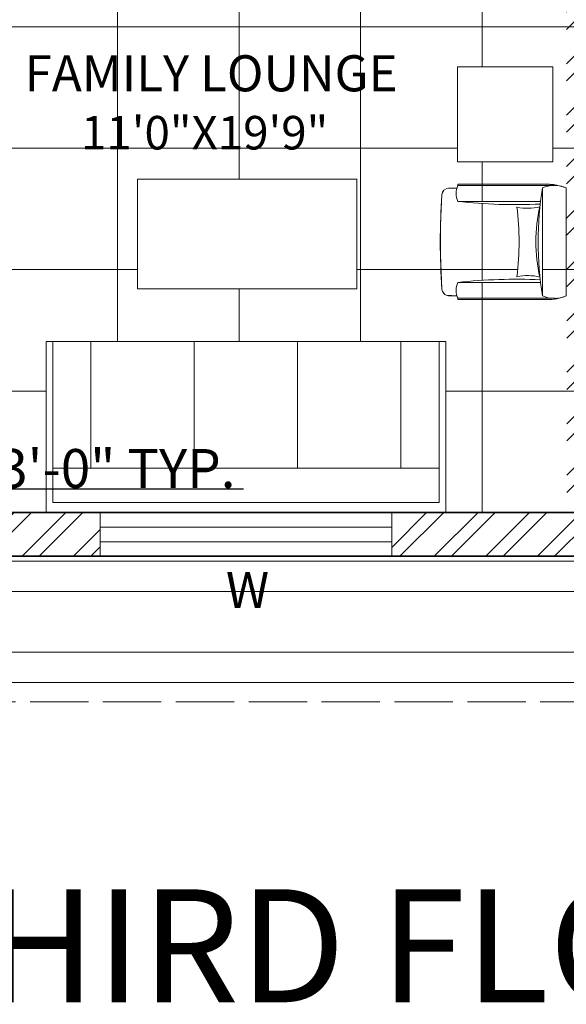
# Model space of a CAD drawing. Units: inches. Extents: x 351 to 1738, y -265 to 286.
# Tile 20 of 38: x 1268 to 1380, y -265 to -63. Entities that reach past the tile are written whole.
import ezdxf

# ---------------------------------------------------------------- set-up
doc = ezdxf.new("R2010")
doc.units = ezdxf.units.IN
doc.header["$MEASUREMENT"] = 0
doc.linetypes.add('ACAD_ISO02W100', pattern=[15, 12, -3])
for name, color, linetype, lineweight in [('A-ANNO-DIMS', 2, 'Continuous', 18), ('A-ANNO-SYMB', 7, 'Continuous', 18), ('A-ANNO-TITL', 7, 'Continuous', 35), ('A-AREA-IDEN', 7, 'Continuous', 18), ('A-FLOR-OVHD', 1, 'ACAD_ISO02W100', 18), ('A-FLOR-PATT', 9, 'Continuous', 9), ('A-FURN', 18, 'Continuous', 13), ('A-GLAZ', 4, 'Continuous', 18), ('A-WALL', 7, 'Continuous', 35), ('A-WALL-PATT', 152, 'Continuous', 13)]:
    doc.layers.add(name, color=color, linetype=linetype, lineweight=lineweight)
doc.styles.add('Annotative', font='arial.ttf')
doc.styles.get("Standard").update_dxf_attribs({"font": 'arial.ttf'})
doc.dimstyles.get("Standard").update_dxf_attribs({"dimtxt": 8, "dimasz": 5, "dimexe": 0.18, "dimexo": 0.0625, "dimgap": 0.09, "dimtad": 1, "dimtoh": 1, "dimzin": 0, "dimdsep": 46, "dimlunit": 4, "dimtxsty": 'Standard', "dimcen": 0, "dimclre": 256, "dimadec": 0, "dimazin": 0, "dimtfac": 1, "dimtofl": 0, "dimtmove": 0, "dimatfit": 3, "dimfxl": 1, "dimtolj": 1, "dimtzin": 0, "dimlwe": -1, "dimarcsym": 0})

# ---------------------------------------------------------------- blocks, each defined once
blk = doc.blocks.new('TABLE-COFFEE-RECT')
blk.add_lwpolyline([(0, 0), (0, 22.55), (45.11, 22.55), (45.11, 0)], close=True)
blk = doc.blocks.new('WIN-60')
for p, q in [((0, 6), (60, 6)), ((0, 3), (60, 3))]:
    blk.add_line(p, q)
blk.add_lwpolyline([(60, 0), (60, 9), (0, 9), (0, 0)], close=True)
blk = doc.blocks.new('*D38')
at = {"layer": 'A-ANNO-DIMS', "color": 0, "lineweight": -2, "transparency": 16777216}
for p, q in [((1215.46, -164.13), (1215.46, -159.13)), ((1215.46, -159.13), (1313.61, -159.13)), ((1215.46, -195.23), (1215.46, -169.13))]:
    blk.add_line(p, q, dxfattribs=at)
at = {"layer": 'A-ANNO-DIMS', "transparency": 16777216}
for p, q in [((1210.11, -164.13), (1215.64, -164.13)), ((1210.11, -200.23), (1215.64, -200.23))]:
    blk.add_line(p, q, dxfattribs=at)
at = {"layer": 'A-ANNO-DIMS', "color": 0, "transparency": 16777216}
for points in [[(1214.63, -169.13), (1216.3, -169.13), (1215.46, -164.13)], [(1214.63, -195.23), (1216.3, -195.23), (1215.46, -200.23)]]:
    blk.add_solid(points, dxfattribs=at)
at = {"layer": 'Defpoints', "color": 0, "transparency": 16777216}
for p in [(1210.05, -164.13), (1215.46, -164.13), (1210.05, -200.23)]:
    blk.add_point(p, dxfattribs=at)
at = {"layer": 'A-ANNO-DIMS', "color": 0, "transparency": 16777216, "insert": (1264.58, -154.96), "char_height": 8, "attachment_point": 5}
blk.add_mtext('\\A1;PLANT B 3\'-0" TYP.', dxfattribs=at)

msp = doc.modelspace()

# ---------------------------------------------------------------- hatches: boundary and pattern name
at = {"layer": 'A-FLOR-PATT', "transparency": 33554559}
h = msp.add_hatch(dxfattribs=at)
h.set_pattern_fill('ANSI37', color=256, scale=200, angle=135)
h.set_pattern_definition([(180, (1112.704, -164.037), (-2e-15, -25), []), (270, (1112.704, -164.037), (25, -5e-15), [])])
h.paths.add_polyline_path([(1380.064, 73.463), (1380.132, 148.463), (1338.064, 148.463), (1290.704, 148.463), (1290.704, 88.463), (1248.704, 88.463), (1248.704, -2.009), (1244.704, -2.009), (1244.704, 142.457), (1160.704, 142.457), (1160.704, 158.963), (1160.704, 170.137), (1160.704, 206.137), (1160.704, 228.963), (1112.704, 228.963), (1112.704, 209.963), (1112.704, 168.963), (1124.704, 168.963), (1124.704, 162.963), (1112.704, 162.963), (1112.704, 64.463), (1112.704, 60.463), (1112.704, 0.463), (1112.704, -48.026), (1146.804, -47.981), (1146.804, -35.691), (1207.804, -35.691), (1207.804, -47.902), (1236.542, -47.864), (1236.544, -50.009), (1248.5, -50.009), (1248.506, -102.915), (1248.512, -150.915), (1248.514, -164.037), (1248.549, -164.037), (1273.017, -164.037), (1273.017, -128.799), (1355.24, -128.799), (1355.24, -164.037), (1384.204, -164.037), (1384.204, -57.037), (1380.064, -57.037), (1380.064, -48.037), (1392.064, -48.037), (1392.064, -53.037), (1406.549, -53.037), (1406.549, -57.037), (1401.204, -57.037), (1401.204, -147.037), (1468.204, -147.037), (1468.204, -138.5), (1472.204, -138.5), (1472.204, -102.5), (1468.204, -102.5), (1468.204, -57.037), (1442.549, -57.037), (1442.549, -53.037), (1463.049, -53.037), (1463.049, -40.747), (1524.049, -40.747), (1524.049, -48.037), (1536.064, -48.037), (1536.064, -53.037), (1557.704, -53.037), (1557.704, 204.963), (1384.204, 204.963), (1384.204, 73.463), (1392.064, 73.463), (1392.064, 64.463), (1384.204, 64.463), (1384.204, -3.5), (1380.204, -3.537), (1380.204, 64.463), (1380.064, 64.463)])
h.paths.add_polyline_path([(1510.714, 86.458, -0.1039845), (1511.661, 85.595, 0.4704384), (1510.158, 87.614, 0.0961001)], flags=16)
h.paths.add_polyline_path([(1510.443, 100.266, 0.009798), (1504.693, 100.48, 0.0287898), (1504.6, 99.767, -0.1653311), (1505.519, 96.135, -0.1436014)], flags=16)
h.paths.add_polyline_path([(1487.201, 85.595, -0.1039845), (1488.148, 86.458, 0.0961001), (1488.704, 87.614, 0.4704384)], flags=0)
h.paths.add_polyline_path([(1495.052, 100.43), (1494.178, 100.43, -0.0264629), (1494.262, 99.774, -0.1442193)], flags=16)
h.paths.add_polyline_path([(1444.485, 86.458, -0.1039845), (1445.433, 85.595, 0.4704384), (1443.93, 87.614, 0.0961001)], flags=16)
h.paths.add_polyline_path([(1420.972, 85.595, -0.1039845), (1421.92, 86.458, 0.0961001), (1422.475, 87.614, 0.4704384)], flags=16)
h.paths.add_polyline_path([(1428.632, 100.335, 0.0010541), (1427.971, 100.309, -0.0215241), (1428.033, 99.774, -0.1143008)], flags=16)
h.paths.add_polyline_path([(1419.906, 143.708, 0.0249793), (1420.222, 157.526), (1421.573, 159.101), (1421.573, 175.369), (1391.393, 175.369), (1391.393, 200.519), (1542.294, 200.519), (1542.294, 175.369), (1512.028, 175.369, 0.0198653), (1511.521, 153.838, 0.0251335), (1512.758, 118.323, 0.0205529), (1512.942, 115.253), (1419.834, 115.253, -0.0004142), (1419.843, 124.798), (1413.059, 124.798), (1413.059, 84.437, -0.0618528), (1415.831, 80.45, -0.0930773), (1420.972, 85.595, -0.2675367), (1422.371, 84.732, 0.0851103), (1424.052, 84.616, -0.8853927), (1424.033, 84.851, -1.1258145), (1424.073, 84.366, -0.0879871), (1422.371, 84.732, -0.2675367), (1422.326, 83.089, -0.3705421), (1420.972, 85.595, 0.0930773), (1415.831, 80.45, -0.0874142), (1417.914, 73.937), (1418.941, 73.937, 0.0272504), (1418.913, 76.906, -0.1157032), (1421.051, 73.937), (1445.354, 73.937, -0.1157032), (1447.492, 76.906, 0.0272504), (1447.464, 73.937), (1448.491, 73.937, -0.0874142), (1450.574, 80.45, 0.0930773), (1445.433, 85.595, -0.3705421), (1444.079, 83.089, -0.2675367), (1444.034, 84.732, -0.0879871), (1442.332, 84.366, -1.1258145), (1442.372, 84.851, -2.0327363), (1442.364, 84.368, 0.0863779), (1444.034, 84.732, -0.2675367), (1445.433, 85.595, -0.0930773), (1450.574, 80.45, -0.2577317), (1466.483, 90.927, -0.4786702), (1468.832, 91.907, -0.4786702), (1471.18, 90.927, -0.26264), (1483.053, 81.78, -0.0718662), (1487.201, 85.595, -0.2675367), (1488.6, 84.732, 0.0851103), (1490.28, 84.616, -0.8853927), (1490.262, 84.851, -1.1258145), (1490.301, 84.366, -0.0879871), (1488.6, 84.732, -0.2675367), (1488.554, 83.089, -0.3705421), (1487.201, 85.595, 0.0718662), (1483.053, 81.78, -0.1320648), (1484.143, 73.937), (1485.169, 73.937, 0.0272504), (1485.142, 76.906, -0.1157032), (1487.28, 73.937), (1511.582, 73.937, -0.1157032), (1513.72, 76.906, 0.0272504), (1513.693, 73.937), (1514.719, 73.937, -0.0874142), (1516.802, 80.45, 0.0930773), (1511.661, 85.595, -0.3705421), (1510.308, 83.089, -0.2675367), (1510.262, 84.732, -0.0879871), (1508.561, 84.366, -1.1258145), (1508.601, 84.851, -2.0327363), (1508.592, 84.368, 0.0863779), (1510.262, 84.732, -0.2675367), (1511.661, 85.595, -0.0930773), (1516.802, 80.45, -0.0618528), (1519.575, 84.437), (1519.575, 73.937), (1413.059, 73.937), (1413.059, 124.798), (1419.843, 124.798, -0.0008205)], flags=16)
h.paths.add_polyline_path([(1220.149, 54.133, -0.1039845), (1220.869, 53.476, 0.4704384), (1219.727, 55.011, 0.0961001)], flags=16)
h.paths.add_polyline_path([(1219.944, 64.626, 0.009798), (1215.574, 64.789, 0.0287898), (1215.503, 64.247, -0.1653311), (1216.201, 61.487, -0.1436014)], flags=16)
h.paths.add_polyline_path([(1209.779, 64.449, 0.0974459), (1209.339, 64.751), (1208.247, 64.751, 0.1273905), (1207.7, 64.326, 0.1715858), (1206.95, 61.475, -0.1588542), (1207.636, 59.45, 0.0158984), (1207.795, 59.218, 0.0615457), (1208.598, 59.616, 0.1754158), (1208.638, 60.099, -0.2847793), (1209.348, 62.472, 0.3262165)], flags=16)
h.paths.add_polyline_path([(1169.818, 54.133, -0.1039845), (1170.538, 53.476, 0.4704384), (1169.396, 55.011, 0.0961001)], flags=16)
h.paths.add_polyline_path([(1159.017, 62.472, 0.2847642), (1158.307, 60.099, -0.1754332), (1158.267, 59.616, 0.3929302), (1159.448, 64.449, -0.3262298)], flags=16)
h.paths.add_polyline_path([(1156.342, 58.239, -0.1783213), (1154.011, 55.31, -0.1747359), (1154.722, 55.233, -0.2008015), (1156.27, 56.086, 0.1269899), (1157.283, 58.991, -0.0912053)], flags=16)
h.paths.add_polyline_path([(1156.624, 61.413, 0.1572752), (1157.316, 64.247, 0.1696217)], flags=16)
h.paths.add_polyline_path([(1152.67, 54.133, -0.0961001), (1151.95, 53.476, 0.0640762), (1154.465, 54.384, 0.1990158)], flags=16)
h.paths.add_polyline_path([(1202.281, 53.476, -0.1039845), (1203, 54.133, 0.0961001), (1203.423, 55.011, 0.4704384)], flags=0)
h.paths.add_polyline_path([(1151.139, 97.64, 0.0249793), (1151.379, 108.141), (1152.406, 109.338), (1152.406, 121.701), (1129.47, 121.701), (1129.47, 140.814), (1244.149, 140.814), (1244.149, 121.701), (1221.148, 121.701, 0.0198653), (1220.763, 105.338, 0.0251335), (1221.703, 78.349, 0.0205529), (1221.843, 76.016), (1151.078, 76.016, -0.1287433), (1148.786, 65.037, 0.5393525), (1150.327, 64.171, -0.027594), (1163.481, 64.751, 0.0976954), (1163.04, 64.449, 0.3262165), (1163.471, 62.472, -0.2847765), (1164.181, 60.099, -0.1947567), (1165.846, 61.443, -0.1554021), (1165.172, 64.247, -0.1660224), (1165.869, 61.475, -0.1770142), (1167.852, 62.77, -0.4482027), (1169.974, 60.807, -0.3934987), (1167.679, 57.86, -0.8955483), (1168.438, 54.524, -0.3557668), (1166.218, 56.086, -0.066024), (1165.505, 57.539), (1165.251, 56.243, -0.3717324), (1164.02, 59.758, -0.3736141), (1163.04, 64.449, -0.0976954), (1163.481, 64.751, 0.0213538), (1153.294, 64.429, -0.1341826), (1156.695, 61.368, 0.1868727), (1154.636, 62.77, 0.4482027), (1152.514, 60.807, 0.4037263), (1154.905, 57.846, 0.7112192), (1153.334, 55, 0.5315397), (1151.95, 53.476, -0.2675367), (1153.013, 52.821, 0.0851103), (1154.29, 52.732, -0.8853927), (1154.276, 52.911, -1.1258145), (1154.306, 52.543, -0.0879871), (1153.013, 52.821, -0.2675367), (1152.978, 51.572, -0.3705421), (1151.95, 53.476, 0.0930773), (1148.043, 49.566, -0.0874142), (1149.626, 44.617), (1150.406, 44.617, 0.0272504), (1150.385, 46.873, -0.1157032), (1152.01, 44.617), (1170.478, 44.617, -0.1157032), (1172.103, 46.873, 0.0272504), (1172.082, 44.617), (1172.862, 44.617, -0.0874142), (1174.445, 49.566, 0.0930773), (1170.538, 53.476, -0.3705421), (1169.51, 51.572, -0.2675367), (1169.475, 52.821, -0.0879871), (1168.182, 52.543, -1.1258145), (1168.212, 52.911, -2.0327363), (1168.206, 52.544, 0.0863779), (1169.475, 52.821, -0.2675367), (1170.538, 53.476, -0.0930773), (1174.445, 49.566, -0.2577317), (1186.536, 57.528, -0.4786702), (1188.321, 58.273, -0.4786702), (1190.106, 57.528, -0.26264), (1199.128, 50.577, -0.0718662), (1202.281, 53.476, -0.2675367), (1203.344, 52.821, 0.0851103), (1204.621, 52.732, -0.8853927), (1204.607, 52.911, -1.1258145), (1204.637, 52.543, -0.0879871), (1203.344, 52.821, -0.2675367), (1203.309, 51.572, -0.3705421), (1202.281, 53.476, 0.0718662), (1199.128, 50.577, -0.1320648), (1199.957, 44.617), (1200.737, 44.617, 0.0272504), (1200.716, 46.873, -0.1157032), (1202.341, 44.617), (1220.809, 44.617, -0.1157032), (1222.434, 46.873, 0.0272504), (1222.413, 44.617), (1223.193, 44.617, -0.0874142), (1224.776, 49.566, 0.0930773), (1220.869, 53.476, -0.3705421), (1219.841, 51.572, -0.2675367), (1219.806, 52.821, -0.0879871), (1218.513, 52.543, -1.1258145), (1218.543, 52.911, -2.0327363), (1218.537, 52.544, 0.0863779), (1219.806, 52.821, -0.2675367), (1220.869, 53.476, -0.0930773), (1224.776, 49.566, -0.0618528), (1226.883, 52.597), (1226.883, 44.617), (1145.936, 44.617), (1145.936, 83.269), (1151.091, 83.269, -0.0008205)], flags=16)
h.paths.add_polyline_path([(1218.01, 57.86, -0.8955483), (1218.769, 54.524, -0.3557668), (1216.549, 56.086, -0.066024), (1215.836, 57.539), (1215.582, 56.243, -0.3717324), (1214.351, 59.758, -0.3736141), (1213.371, 64.449, 0.3262165), (1213.802, 62.472, -0.2847765), (1214.512, 60.099, -0.1947567), (1216.177, 61.443, -0.1799907), (1218.183, 62.77, -0.4482027), (1220.305, 60.807, -0.3934987)], flags=16)
h.paths.add_polyline_path([(1424.735, 91.363, -0.3934987), (1421.715, 95.241, -0.4482027), (1424.507, 97.824, -0.1799907), (1427.147, 96.077, -0.1947567), (1429.338, 94.309, -0.2847765), (1430.272, 97.432, 0.3262165), (1430.839, 100.034, -0.3736141), (1429.55, 93.861, -0.3717324), (1427.929, 89.235), (1427.596, 90.941, -0.066024), (1426.657, 89.029, -0.3557668), (1423.736, 86.973, -0.8955483)], flags=16)
h.paths.add_polyline_path([(1238.033, 131.257, -1), (1227.329, 131.257, -1)], flags=0)
h.paths.add_polyline_path([(1235.357, 131.257, -1), (1230.005, 131.257, -1)], flags=0)
h.paths.add_polyline_path([(1214.039, 54.243, 0.1543819), (1214.38, 53.992, 0.3589549), (1213.613, 54.016, 0.6039484), (1214.379, 53.657, 0.3713191), (1213.968, 52.872, 0.1879935), (1214.312, 52.809, -0.592455), (1213.953, 52.967, -0.2942791), (1214.083, 53.691, -1.3001871), (1213.881, 54.134, -0.2837621), (1214.469, 53.896, 1.1509396)], flags=16)
h.paths.add_polyline_path([(1212.091, 56.286, -0.4084338), (1211.337, 56.445, -0.0362594), (1211.098, 56.848, -0.2360976), (1211.59, 56.63, 0.0353445), (1211.835, 56.543, -0.4752408), (1212.091, 56.286, -0.4752408), (1212.438, 56.182, 0.0353445), (1212.631, 56.007, -0.2360976), (1213.056, 55.676, -0.0362594), (1212.588, 55.697, -0.4084338)], flags=16)
h.paths.add_polyline_path([(1211.469, 50.297, 0.296043), (1210.47, 50.527, 0.310883), (1211.931, 50.148, 0.0212546)], flags=16)
h.paths.add_polyline_path([(1213.739, 51.818, -0.0362594), (1213.271, 51.838, -0.4084337), (1212.774, 52.427, -0.0947856), (1212.293, 50.703, 1.1504738), (1212.911, 50.232, 0.1662877), (1213.265, 50.68, -0.0252543), (1212.603, 50.13, 1.0879317), (1212.471, 49.407, 0.1662877), (1213.02, 49.251, -0.016128), (1212.567, 49.563, -0.286859), (1212.217, 49.638, 0.0221563), (1212.046, 50.055, -0.6461302), (1212.185, 50.498, 0.0884116), (1212.732, 52.077, -1.1860374), (1213.121, 52.323, 0.0353445), (1213.314, 52.148, -0.2360976)], flags=16)
h.paths.add_polyline_path([(1212.094, 50.342, -0.0485241), (1211.54, 49.605, -1.1038339), (1211.397, 48.738, -0.7855147), (1211.683, 48.254, -0.3920429), (1210.948, 48.525, -0.3928194), (1210.561, 47.995, -0.592455), (1210.201, 48.153, -0.2942791), (1210.331, 48.877, -0.7041716), (1210.316, 49.592, -0.6793441), (1210.729, 50.112, 0.5636764)], flags=16)
h.paths.add_polyline_path([(1211.274, 49.829, -0.1398258), (1210.745, 49.859, -0.2178785), (1210.948, 49.509, -0.4985724)], flags=0)
h.paths.add_polyline_path([(1433.426, 81.49, -0.181571), (1434.245, 81.788, -0.0080665), (1433.726, 82.205, 0.0455784), (1432.755, 81.242, 0.1790113)], flags=16)
h.paths.add_polyline_path([(1434.146, 81.009, -0.1324418), (1433.645, 80.771, 0.2590893), (1433.234, 80.471, -0.1802109), (1433.392, 80.805, -0.1699398), (1432.758, 81.109, 0.0326525), (1433.273, 80.474, -0.4933627), (1434.046, 80.146, -0.3904966)], flags=16)
h.paths.add_polyline_path([(1434.83, 80.047, -0.9475376), (1435.294, 79.576, -0.2991282), (1434.625, 79.404, -0.2704392), (1435.01, 78.591, -0.592455), (1434.537, 78.382, -0.3928194), (1434.027, 79.08, -0.3920429), (1433.06, 78.723, -0.3520423), (1433.003, 79.197, -0.1972159), (1433.75, 79.734, -0.7136405), (1434.447, 79.939, -0.2147903), (1434.819, 80.475, 0.4088333), (1435.075, 80.803, -0.2261519)], flags=16)
h.paths.add_polyline_path([(1432.67, 81.217, -0.4542182), (1431.897, 79.923, -0.4144105), (1431.301, 80.035, 0.0161291), (1431.897, 80.445, 0.2795702), (1432.073, 80.871, -0.2895037), (1431.103, 81.321, -0.4144105), (1430.978, 81.915, 0.0161296), (1431.586, 81.521, 0.341293), (1432.125, 81.583, -0.8131856)], flags=16)
h.paths.add_polyline_path([(1429.893, 86.381, -0.9475376), (1430.358, 85.91, -0.1731062), (1429.984, 85.712, -0.0388172), (1431.625, 84.214, -0.0879005), (1432.097, 88.549, -0.0497684), (1431.254, 88.49, -0.2360976), (1431.814, 88.925, 0.0353445), (1432.067, 89.155, -0.4752408), (1432.524, 89.291, -0.4752408), (1432.86, 89.63, 0.0353445), (1433.182, 89.744, -0.2360976), (1433.83, 90.032, -0.0362594), (1433.516, 89.502, -0.4084338), (1432.524, 89.291, -0.3124239), (1432.106, 88.58, 0.0885594), (1431.625, 84.214, -0.4084337), (1430.971, 83.439, -0.0362594), (1430.355, 83.412, -0.2360976), (1430.914, 83.847, 0.0353445), (1431.168, 84.078, -0.4752408), (1431.625, 84.214, 0.0388172), (1429.984, 85.712, -0.3217316), (1429.333, 86.048, -0.32743), (1429.883, 86.809, 0.4088333), (1430.138, 87.138, -0.2261519)], flags=16)
h.paths.add_polyline_path([(1211.206, 58.616, -0.9997836), (1211.336, 59.323, -0.6149935)], flags=16)
h.paths.add_polyline_path([(1210.288, 49.429, 0.1543819), (1210.629, 49.178, 0.3589549), (1209.861, 49.202, 0.6039484), (1210.627, 48.843, -0.5348247), (1210.806, 49.295, 0.7483464)], flags=16)
h.paths.add_polyline_path([(1209.589, 51.828, -0.0087906), (1209.775, 51.753, 0.1122315), (1209.466, 52.019, 1.4188509), (1209.014, 51.708, -0.4587257), (1208.651, 51.073, -0.592455), (1208.291, 51.232, -0.2942791), (1208.421, 51.955, -1.3001871), (1208.219, 52.398, -0.2260052), (1208.719, 52.257, -0.4755189), (1209.158, 52.369, -1.4554994), (1209.603, 52.664, 0.4213049), (1209.191, 52.262, -0.5912116), (1208.979, 51.796, 0.4973986), (1209.773, 51.333, 0.6493116)], flags=16)
h.paths.add_polyline_path([(1208.029, 52.041, 0.5446671), (1208.832, 52.045, 0.220132)], flags=0)
h.paths.add_polyline_path([(1210.438, 51.425, -0.2041997), (1210.277, 52.018, 0.2708262), (1209.915, 52.897, 0.3241145)], flags=0)
h.paths.add_polyline_path([(1209.668, 52.407, -0.60139), (1208.99, 52.221, -0.3949159), (1208.248, 52.83, -0.8367916), (1208.651, 53.017, -0.3384876), (1209.039, 52.571, 0.1941379), (1209.191, 52.262, 0.4139945), (1209.712, 52.475, 0.5177103), (1210.503, 51.416, 0.401922), (1209.493, 50.93, 0.2063956), (1209.516, 50.165, -0.3194629), (1210.417, 51.418, -0.466635)], flags=16)
h.paths.add_polyline_path([(1206.601, 56.086, -0.3557668), (1204.381, 54.524, -0.9211983), (1205.236, 57.846, 0.2065693), (1207.614, 58.991, -0.1269899)], flags=16)
h.paths.add_polyline_path([(1435.487, 82.816, 0.5277653), (1436.615, 83.361, 0.5085402), (1437.05, 82.433, 0.592455), (1437.524, 82.641, 0.3312448), (1436.963, 83.548, 0.3878632), (1437.808, 83.626, 0.5929544), (1437.618, 84.176, 0.2260158), (1436.961, 83.99, 0.3182053), (1437.588, 84.854, 0.6893744), (1437.05, 84.991, 0.3357648), (1436.539, 84.41, -0.1569934), (1436.404, 84.065, -0.4346112), (1436.961, 83.99, -0.2147903), (1437.333, 84.526, 0.4088333), (1437.588, 84.854, -0.2261519), (1437.343, 84.097, -0.9475376), (1437.808, 83.626, -0.2991282), (1437.139, 83.455, -0.2704392), (1437.524, 82.641, -0.592455), (1437.05, 82.433, -0.3928194), (1436.541, 83.13, -0.4396601), (1435.475, 82.794, -0.174614), (1435.942, 82.244, -0.2063956), (1435.912, 81.237, -0.2708262), (1435.125, 82.208, 0.2079765), (1434.686, 82.904, -0.1964955)], flags=16)
h.paths.add_polyline_path([(1435.386, 84.832, 0.270811), (1434.91, 83.676, -0.2042174), (1434.699, 82.895, 0.3241145)], flags=0)
h.paths.add_polyline_path([(1435.68, 84.18, -0.2176564), (1435.554, 83.304, -0.1767045), (1436.236, 83.778, -0.3730364)], flags=0)
h.paths.add_polyline_path([(1435.566, 100.034, 0.3262165), (1436.133, 97.432, -0.2847765), (1437.067, 94.309, -0.1947567), (1439.258, 96.077, -0.1554021), (1438.371, 99.767, -0.1660224), (1439.289, 96.12, -0.1770142), (1441.897, 97.824, -0.4482027), (1444.69, 95.241, -0.3934987), (1441.67, 91.363, -0.8955483), (1442.669, 86.973, -0.3557668), (1439.748, 89.029, -0.066024), (1438.809, 90.941), (1438.476, 89.235, -0.3717324), (1436.855, 93.861, -0.3736141)], flags=16)
h.paths.add_polyline_path([(1191.252, 49.507, -0.2740221), (1190.658, 48.409, 0.2675367), (1191.311, 47.344, 0.3705421)], flags=0)
h.paths.add_polyline_path([(1190.301, 49.717, 0.1990158), (1188.619, 49.04, 0.0640762), (1191.252, 49.507, -0.0961001)], flags=0)
h.paths.add_polyline_path([(1189.518, 47.857, 1.1258145), (1189.676, 47.523, 2.0446052)], flags=0)
h.paths.add_polyline_path([(1464.974, 80.372, 0.2740221), (1465.756, 78.927, -0.0830131)], flags=0)
h.paths.add_polyline_path([(1464.974, 80.372, 0.3705421), (1464.897, 77.525, 0.5763244)], flags=0)
h.paths.add_polyline_path([(1464.974, 80.372, -0.4704384), (1467.284, 81.372, -0.0961001), (1466.226, 80.648, -0.1990158), (1468.439, 79.757, -0.0640762)], flags=0)
h.paths.add_polyline_path([(1189.511, 56.43, -0.2594668), (1188.321, 56.391, -0.2594668), (1187.13, 56.43, 0.0851103), (1188.193, 55.716, -0.8853927), (1188.27, 55.878, -1.1960133), (1188.355, 55.442, 0.1014587)], flags=0)
h.paths.add_polyline_path([(1188.321, 57.596, 0.0780722), (1187.678, 57.24, 0.0155503), (1188.321, 57.136, 0.0155503), (1188.964, 57.24, 0.0780722)], flags=0)
h.paths.add_polyline_path([(1190.164, 55.365, -0.5763244), (1190.106, 57.528, -0.1982945), (1188.321, 58.319, -0.1982945), (1186.536, 57.528, -0.5763244), (1186.477, 55.365, -0.3705421), (1186.536, 57.528, 0.1982945), (1188.321, 58.319, 0.1982945), (1190.106, 57.528, -0.3705421)], flags=0)
h.paths.add_polyline_path([(1188.372, 55.878, 1.1258145), (1188.529, 55.544, 2.0446052)], flags=0)
h.paths.add_polyline_path([(1186.341, 49.717, -0.0961001), (1185.389, 49.507, 0.0640762), (1188.022, 49.04, 0.1990158)], flags=0)
h.paths.add_polyline_path([(1185.389, 49.507, -0.2675367), (1185.984, 48.409, 0.0851103), (1187.046, 47.695, -0.8853927), (1187.123, 47.857, -1.1258145), (1186.966, 47.523, -0.0879871), (1185.984, 48.409, -0.2675367), (1185.331, 47.344, -0.3705421)], flags=0)
h.paths.add_polyline_path([(1399.441, 187.944, -1), (1413.525, 187.944, -1)], flags=0)
h.paths.add_polyline_path([(1402.962, 187.944, -1), (1410.004, 187.944, -1)], flags=0)
h.paths.add_polyline_path([(1357.663, -72.245), (1377.272, -72.245), (1377.272, -91.854), (1357.663, -91.854)], flags=16)
h.paths.add_polyline_path([(1467.256, 78.201, -1.1258145), (1467.049, 77.761, -2.0446052)], flags=0)
h.paths.add_polyline_path([(1468.822, 88.714, 0.9411249), (1469.106, 88.316, 1.1371523), (1468.765, 88.755, 0.890986), (1468.99, 88.245, 0.0948283), (1470.398, 89.481, -0.2675367), (1471.18, 90.927, -0.0281232), (1469.678, 90.547, -0.0287737), (1469.948, 90.311, -0.0203267), (1468.832, 90.41, -0.0203267), (1467.716, 90.311, -0.0287737), (1467.986, 90.547, -0.0281232), (1466.483, 90.927, -0.2675367), (1467.265, 89.481, 0.0851103), (1468.663, 88.542, -1.2023159)], flags=0)
h.paths.add_polyline_path([(1178.25, 124.523, -0.1199286), (1165.65, 124.145, -0.1073492), (1159.133, 124.446, -0.1028906), (1159.132, 130.465, -0.0748968), (1158.993, 137.956, 0.002027), (1167.844, 137.479, -0.07553), (1180.337, 137.666, -0.0758613), (1186.502, 137.688, -0.1409896), (1186.272, 130.046, -0.0954805), (1186.729, 124.748, -0.10603)], flags=0)
h.paths.add_polyline_path([(1469.225, 79.757, -0.1990158), (1471.437, 80.648, -0.0961001), (1470.379, 81.372, -0.4704384), (1472.689, 80.372, -0.3705421), (1472.766, 77.525, -0.2675367), (1471.907, 78.927, -0.0879863), (1470.615, 77.761, -1.1258491), (1470.408, 78.201, -2.0327363), (1470.642, 77.778, 0.0863779), (1471.907, 78.927, -0.2675367), (1472.689, 80.372, -0.0640762)], flags=0)
h.paths.add_polyline_path([(1430.423, 186.902, -0.0748968), (1430.24, 196.758, 0.002027), (1441.887, 196.131, -0.07553), (1458.326, 196.377, -0.0758613), (1466.438, 196.406, -0.1409896), (1466.136, 186.35, -0.0954805), (1466.737, 179.378, -0.10603), (1455.58, 179.082, -0.1199286), (1439, 178.585, -0.1073492), (1430.425, 178.981, -0.1028906)], flags=0)
h.paths.add_polyline_path([(1162.258, 49.939, 0.3357645), (1161.87, 49.497, -0.1569936), (1161.767, 49.235, -0.4346112), (1162.19, 49.178, -0.2147903), (1162.473, 49.585, 1.5291948)], flags=16)
h.paths.add_polyline_path([(1161.683, 49.021, 0.5815181), (1161.268, 49.583, 0.5927609)], flags=16)
h.paths.add_polyline_path([(1162.602, 48.058, 0.3713191), (1162.192, 48.843, 0.4345332), (1162.88, 48.962, 0.1850806), (1162.197, 48.926, 1.1218369)], flags=16)
h.paths.add_polyline_path([(1161.443, 48.941, -1.3071038), (1161.495, 48.571, -0.2177521), (1161.136, 48.254, 0.6973029), (1161.871, 49.048, 0.1215141)], flags=16)
h.paths.add_polyline_path([(1162.531, 49.429, -0.2070837), (1162.05, 49.146, -0.9920299)], flags=16)
h.paths.add_polyline_path([(1161.304, 49.578, -0.7196675), (1161.513, 50.079, -0.1304275), (1160.836, 50.168, 0.0395926)], flags=0)
h.paths.add_polyline_path([(1162.036, 50.584, -0.0080665), (1161.642, 50.9, 0.0293675), (1161.35, 50.297, -0.2057884)], flags=16)
h.paths.add_polyline_path([(1162.882, 51.392, -0.1247327), (1162.763, 51.828, -0.1011907), (1162.399, 51.438, -0.153425)], flags=0)
h.paths.add_polyline_path([(1164.235, 51.85, -0.3091075), (1164.513, 51.136, -0.6271245), (1163.781, 51.603, -0.6859091), (1162.777, 51.219, -0.2332851), (1163.303, 50.165, -0.2708262), (1162.705, 50.903, 0.2041997), (1162.381, 51.425, 0.204182), (1162.542, 52.018, -0.2708414), (1162.903, 52.897, -0.1272607), (1163.219, 52.529, -1.1686811), (1163.781, 52.587, -0.3291117), (1164.168, 53.017, -0.8367917), (1164.571, 52.83, -0.1933406), (1164.391, 52.338, -0.9475376), (1164.744, 51.981, -0.2991282)], flags=16)
h.paths.add_polyline_path([(1163.598, 51.937, -1.2629561), (1163.236, 51.831, 0.0125754), (1162.971, 51.721, 0.2306566), (1163.151, 52.407, -0.1648982), (1163.178, 52.661, -0.4493201), (1163.628, 52.262, -0.721477), (1164.154, 52.088, -0.8499982)], flags=0)
h.paths.add_polyline_path([(1161.613, 58.616, -0.9804131), (1161.525, 59.049, -2.9089348)], flags=16)
h.paths.add_polyline_path([(1160.252, 49.166, -0.4144105), (1159.799, 49.251, 0.0161291), (1160.252, 49.563, 0.2795702), (1160.386, 49.887, -0.2895037), (1159.649, 50.229, -0.4144105), (1159.554, 50.68, 0.0161296), (1160.015, 50.381, 0.6178854), (1160.526, 50.703, -0.0947856), (1160.045, 52.427, -0.1404436), (1159.682, 52.042, -0.0578559), (1159.3, 51.872, 0.5448433), (1160.046, 52.419, -0.0881216), (1160.404, 55.721, -0.0497684), (1159.763, 55.676, -0.2360976), (1160.188, 56.007, 0.0353445), (1160.381, 56.182, -0.4752408), (1160.728, 56.286, -0.4752408), (1160.984, 56.543, 0.0353445), (1161.229, 56.63, -0.2360976), (1161.721, 56.848, -0.0362594), (1161.482, 56.445, -0.4084338), (1160.728, 56.286, -0.3124239), (1160.411, 55.745, 0.0885594), (1160.045, 52.427, 0.1070813), (1160.634, 50.498, -0.4947977), (1160.839, 50.149, -0.4542182)], flags=16)
h.paths.add_polyline_path([(1160.666, 49.808, -2.0765276), (1160.828, 50.172, 0.0195861)], flags=0)
h.paths.add_polyline_path([(1158.439, 53.992, 0.1543819), (1158.78, 54.243, 0.7483463), (1158.262, 54.109, -0.3382251), (1158.492, 53.839, -0.1708158), (1159.124, 53.779, 0.4957286), (1158.938, 54.134, 0.2260157)], flags=16)
h.paths.add_polyline_path([(1160.045, 52.427, 0.0388172), (1158.798, 53.565, -0.1198178), (1158.574, 53.586, -0.3091075), (1158.851, 52.872, -0.1879935), (1158.506, 52.809, 0.592455), (1158.866, 52.967, 0.3312448), (1158.44, 53.657, 0.2012451), (1158.798, 53.565, -0.034023), (1159.901, 52.578, -0.0442527), (1159.698, 52.323, -0.4752408)], flags=16)
h.paths.add_polyline_path([(1336.926, -95.392), (1336.926, -117.945), (1291.82, -117.945), (1291.82, -95.392)], flags=16)
h.paths.add_polyline_path([(1357.535, -97.244), (1357.726, -96.697, 0.0348443)], flags=16)
h.paths.add_polyline_path([(1376.693, -96.478), (1377.301, -96.5, 0.0314968), (1375.907, -96.424), (1357.726, -96.424)], flags=16)
h.paths.add_polyline_path([(1379.403, -119.667, 0.0267056), (1380.043, -119.439, -0.0152991)], flags=16)
h.paths.add_polyline_path([(1357.726, -120.202), (1357.821, -120.202), (1357.821, -120.201)], flags=16)
h.paths.add_polyline_path([(1354.171, -104.592), (1354.469, -98.672, 0.0111377)], flags=16)
h.paths.add_polyline_path([(1355.058, -119.136), (1354.578, -118.539, 0.1431635)], flags=16)
h.paths.add_polyline_path([(1378.851, -96.821), (1378.85, -96.82), (1378.85, -96.82, -0.0496798), (1380.055, -97.191), (1378.85, -96.82, 0.1500541), (1375.135, -97.188), (1375.136, -119.44, -0.0099698), (1374.747, -116.649), (1357.726, -116.649, 0.1693849), (1357.535, -119.382), (1357.535, -119.382), (1357.535, -119.382, 0.0348176), (1357.726, -119.928), (1357.726, -119.928), (1357.726, -119.929, -0.0348772), (1357.535, -119.382), (1355.507, -119.382), (1355.317, -119.278), (1357.535, -119.382, -0.1693939), (1357.726, -116.649, -0.0391513), (1374.686, -116.113, -0.0020149), (1374.625, -115.546, 0.1153223), (1369.915, -115.474, 0.0609215), (1369.922, -101.154, 0.1151459), (1374.625, -101.079, -0.0020164), (1374.686, -100.513, -0.0391511), (1357.726, -99.977), (1374.747, -99.977, -0.0099633), (1375.135, -97.188), (1375.135, -97.188, -0.1501081)], flags=16)
h.paths.add_polyline_path([(1490.963, 91.363, -0.3934987), (1487.944, 95.241, -0.4482027), (1490.736, 97.824, -0.1799907), (1493.376, 96.077, -0.1947567), (1495.567, 94.309, -0.2847765), (1496.501, 97.432, 0.3262165), (1497.068, 100.034, -0.3736141), (1495.778, 93.861, -0.3717324), (1494.158, 89.235), (1493.824, 90.941, -0.066024), (1492.886, 89.029, -0.3557668), (1489.964, 86.973, -0.8955483)], flags=16)
h.paths.add_polyline_path([(1354.86, -97.658), (1355.316, -97.348, 0.1019112)], flags=16)
h.paths.add_polyline_path([(1497.063, 83.327, 0.1767244), (1496.37, 83.785, -0.4051388), (1496.016, 83.384, 0.4973986), (1497.06, 82.774, 0.6493116), (1496.818, 83.426, -0.0087906)], flags=16)
h.paths.add_polyline_path([(1496.339, 83.783, 0.5927609), (1496.886, 84.522, 0.5815181)], flags=16)
h.paths.add_polyline_path([(1495.11, 82.641, 0.592455), (1495.583, 82.433, 0.6769152), (1495.805, 83.59, 0.3756693)], flags=16)
h.paths.add_polyline_path([(1495.015, 84.176, -0.145057), (1495.301, 84.526, -0.4088333), (1495.045, 84.854, 0.2206292), (1495.381, 84.152, -0.199594), (1495.851, 83.764, -0.5240172), (1494.826, 83.626, -0.5929976)], flags=16)
h.paths.add_polyline_path([(1501.655, 81.915, -0.0161291), (1501.048, 81.521, -0.3927187), (1500.462, 81.37, -0.2106699), (1500.607, 81.142, 0.3066994)], flags=16)
h.paths.add_polyline_path([(1500.11, 89.291, -0.4084338), (1499.118, 89.502, -0.0362594), (1498.803, 90.032, -0.2360976), (1499.451, 89.744, 0.0353445), (1499.774, 89.63, -0.4752408), (1500.11, 89.291, -0.4752408), (1500.567, 89.155, 0.0353445), (1500.82, 88.925, -0.2360976), (1501.379, 88.49, -0.0362594), (1500.763, 88.516, -0.4084338)], flags=16)
h.paths.add_polyline_path([(1498.908, 82.205, -0.0513217), (1500.013, 81.134, -0.5879306), (1500.234, 81.676, 0.1070813), (1501.009, 84.214, -0.03529)], flags=16)
h.paths.add_polyline_path([(1496.93, 83.875, -0.2063956), (1497.247, 84.832, -0.2708262), (1497.724, 83.676, 0.2079765), (1497.944, 82.884, -0.3814554)], flags=16)
h.paths.add_polyline_path([(1496.721, 81.237, 0.2708125), (1497.509, 82.208, -0.2042157), (1497.935, 82.895, 0.3241145)], flags=16)
h.paths.add_polyline_path([(1497.529, 80.125, -0.145057), (1497.814, 80.475, -0.703182), (1498.282, 81.178, -0.1229248), (1497.977, 81.714, -0.2708368), (1499.207, 81.49, 0.2079641), (1499.993, 81.248, -0.2651454), (1499.278, 80.472, 0.3819006), (1498.808, 79.947, -0.3059049), (1498.848, 79.519, 0.4994816), (1498.574, 79.217, -0.4587257), (1498.097, 78.382, -0.592455), (1497.624, 78.591, -0.2704392), (1498.009, 79.404, -0.299116), (1497.34, 79.576, -0.5930157)], flags=16)
h.paths.add_polyline_path([(1500.736, 79.923, 0.4144105), (1501.333, 80.035, -0.3216484), (1500.192, 80.765, 0.0198856), (1499.976, 81.251, 0.4653307)], flags=16)
h.paths.add_polyline_path([(1501.009, 84.214, -0.0388172), (1502.649, 85.712, -0.1730946), (1502.276, 85.91, -0.5930157), (1502.465, 86.46, -0.145057), (1502.751, 86.809, -0.4088333), (1502.495, 87.138, 0.2206292), (1502.831, 86.436, -0.199594), (1503.301, 86.048, -0.3217316), (1502.649, 85.712, 0.0388172), (1501.009, 84.214, 0.1224486), (1501.412, 83.755, 0.4754908), (1501.335, 84.226, 0.055822), (1501.719, 83.847, -0.2360976), (1502.278, 83.412, -0.0362594), (1501.663, 83.439, -0.4084338)], flags=16)
h.paths.add_polyline_path([(1501.794, 100.034, 0.3262165), (1502.362, 97.432, -0.2847765), (1503.295, 94.309, -0.1947567), (1505.486, 96.077, -0.1799907), (1508.126, 97.824, -0.4482027), (1510.918, 95.241, -0.3934987), (1507.899, 91.363, -0.8955483), (1508.898, 86.973, -0.3557668), (1505.976, 89.029, -0.066024), (1505.038, 90.941), (1504.704, 89.235, -0.3717324), (1503.084, 93.861, -0.3736141)], flags=16)
h.paths.add_polyline_path([(1146.29, 131.257, -1), (1135.587, 131.257, -1)], flags=0)
h.paths.add_polyline_path([(1143.614, 131.257, -1), (1138.262, 131.257, -1)], flags=0)
h.paths.add_polyline_path([(1524.064, 73.463), (1536.064, 73.463), (1536.064, 64.463), (1524.064, 64.463)], flags=16)
h.paths.add_polyline_path([(1520.162, 187.944, -1), (1534.246, 187.944, -1)], flags=0)
h.paths.add_polyline_path([(1530.725, 187.944), (1527.204, 187.944), (1527.204, 184.423, 0.4142136)], flags=0)
h.paths.add_polyline_path([(1278.415, -91.154), (1331.067, -91.154), (1331.067, -80.583), (1278.415, -80.583)], flags=24)
h.paths.add_polyline_path([(1266.655, -79.354), (1354.738, -79.354), (1354.738, -67.817), (1266.655, -67.817)], flags=24)
h.paths.add_polyline_path([(1115.482, 206.184), (1155.098, 206.184), (1155.098, 217.714), (1115.482, 217.714)], flags=24)
h.paths.add_polyline_path([(1161.771, 8.501), (1222.466, 8.501), (1222.466, 19.079), (1161.771, 19.079)], flags=24)
h.paths.add_polyline_path([(1164.656, 18.795), (1210.615, 18.795), (1210.615, 30.324), (1164.656, 30.324)], flags=24)
h.paths.add_polyline_path([(1368.147, -32.882), (1379.362, -32.882), (1379.362, -21.733), (1368.147, -21.733)], flags=24)
h.paths.add_polyline_path([(1244.842, -31.012), (1256.057, -31.012), (1256.057, -19.863), (1244.842, -19.863)], flags=24)
h.paths.add_polyline_path([(1114.589, 195.739), (1156.517, 195.739), (1156.517, 206.31), (1114.589, 206.31)], flags=24)
h.paths.add_polyline_path([(1436.398, 37.632), (1505.131, 37.632), (1505.131, 48.203), (1436.398, 48.203)], flags=24)
h.paths.add_polyline_path([(1435.991, 47.919), (1507.906, 47.919), (1507.906, 59.456), (1435.991, 59.456)], flags=24)
h.paths.add_polyline_path([(1415.107, -124.896), (1457.038, -124.896), (1457.038, -114.318), (1415.107, -114.318)], flags=24)
h.paths.add_polyline_path([(1417.992, -114.602), (1457.609, -114.602), (1457.609, -103.073), (1417.992, -103.073)], flags=24)
h = msp.add_hatch(dxfattribs=at)
h.set_pattern_fill('ANSI32', color=256, scale=50, angle=135)
h.set_pattern_definition([(180, (1038.704, -199.037), (-2e-15, -18.75), []), (180, (1032.454, -192.787), (-2e-15, -18.75), [])])
h.paths.add_polyline_path([(1248.506, -102.915), (1236.559, -102.916), (1236.553, -56.864), (1112.704, -57.026), (1112.704, -57.037), (1103.704, -57.037), (1103.704, -45.037), (1103.704, 98.963), (1076.434, 98.963), (1076.549, -81.037), (1071.549, -81.037), (1043.704, -81.037), (1038.704, -81.037), (1038.704, -161.037), (1043.704, -161.037), (1043.704, -173.037), (1038.704, -173.037), (1038.704, -199.037), (1562.704, -199.037), (1562.704, -173.037), (1236.549, -173.037), (1236.549, -164.037), (1236.693, -164.037), (1236.676, -150.916), (1248.512, -150.915)])
h.paths.add_polyline_path([(1236.133, -134.078), (1247.348, -134.078), (1247.348, -122.929), (1236.133, -122.929)], flags=24)
h.paths.add_polyline_path([(1308.144, -185.548), (1321.66, -185.548), (1321.66, -174.4), (1308.144, -174.4)], flags=24)
h.paths.add_polyline_path([(1121.632, -122.88), (1179.647, -122.88), (1179.647, -112.309), (1121.632, -112.309)], flags=24)
h.paths.add_polyline_path([(1124.515, -112.593), (1177.986, -112.593), (1177.986, -101.056), (1124.515, -101.056)], flags=24)
h.paths.add_polyline_path([(1091.374, 23.58), (1104.89, 23.58), (1104.89, 34.728), (1091.374, 34.728)], flags=24)
at = {"layer": 'A-WALL-PATT'}
h = msp.add_hatch(dxfattribs=at)
h.set_pattern_fill('ANSI32', color=256, scale=20)
h.set_pattern_definition([(45, (1034.704, -173.037), (-5.3033, 5.3033), []), (45, (1038.24, -173.037), (-5.3033, 5.3033), [])])
h.paths.add_polyline_path([(1043.704, -57.037), (1034.704, -57.037), (1034.704, -81.037), (1043.704, -81.037)])
h.paths.add_polyline_path([(1043.704, 198.963), (1034.704, 198.963), (1034.704, -45.037), (1043.704, -45.037)])
h.paths.add_polyline_path([(1043.704, 243.963), (1034.704, 243.963), (1034.704, 237.963), (1034.704, 210.963), (1043.704, 210.963)])
h.paths.add_polyline_path([(1112.704, 255.963), (1043.704, 255.963), (1043.704, 246.963), (1103.704, 246.963), (1103.704, 237.963), (1112.704, 237.963), (1112.704, 251.963)])
h.paths.add_polyline_path([(1056.704, 207.963), (1043.704, 207.963), (1043.704, 198.963), (1056.704, 198.963)])
h.paths.add_polyline_path([(1103.704, 207.963), (1092.704, 207.963), (1092.704, 198.963), (1103.704, 198.963)])
h.paths.add_polyline_path([(1112.704, 228.963), (1103.704, 228.963), (1103.704, 74.963), (1112.704, 74.963), (1112.704, 97.5)])
h.paths.add_polyline_path([(1284.129, -164.037), (1248.549, -164.037), (1248.549, -173.037), (1284.129, -173.037)])
h.paths.add_polyline_path([(1524.064, -164.037), (1472.204, -164.037), (1472.204, -138.5), (1468.204, -138.5), (1468.204, -164.037), (1344.129, -164.037), (1344.129, -173.037), (1524.064, -173.037)])
h.paths.add_polyline_path([(1384.204, -57.037), (1380.065, -57.037), (1380.204, -164.037), (1384.204, -164.037)])
h.paths.add_polyline_path([(1566.704, -138), (1557.704, -138), (1557.704, -164.037), (1536.064, -164.037), (1536.064, -173.037), (1566.704, -173.037)])
h.paths.add_polyline_path([(1566.704, -30.189), (1557.704, -30.189), (1557.704, -53.037), (1536.064, -53.037), (1536.064, -57.037), (1557.704, -57.037), (1557.704, -102), (1566.704, -102)])
h.paths.add_polyline_path([(1524.064, -53.037), (1442.549, -53.037), (1442.549, -57.037), (1468.204, -57.037), (1468.204, -102.5), (1472.204, -102.5), (1472.204, -57.037), (1524.064, -57.037)])
h.paths.add_polyline_path([(1566.704, 120.993), (1557.704, 120.993), (1557.704, 29.811), (1566.704, 29.811)])
h.paths.add_polyline_path([(1384.204, 64.463), (1380.204, 64.463), (1380.204, -3.5), (1384.204, -3.5)])
h.paths.add_polyline_path([(1266.549, 237.963), (1248.704, 237.963), (1248.704, 228.963), (1266.549, 228.963)])
h.paths.add_polyline_path([(1329.549, 237.963), (1302.549, 237.963), (1302.549, 228.963), (1329.549, 228.963)])
h.paths.add_polyline_path([(1380.204, 237.963), (1365.549, 237.963), (1365.549, 228.963), (1380.204, 228.963)])
h.paths.add_polyline_path([(1524.064, 237.963), (1392.204, 237.963), (1392.204, 228.963), (1524.064, 228.963)])
h.paths.add_polyline_path([(1384.204, 228.963), (1380.204, 228.963), (1380.204, 73.463), (1384.204, 73.463)])
h.paths.add_polyline_path([(1566.704, 237.963), (1536.064, 237.963), (1536.064, 228.963), (1557.704, 228.963), (1557.704, 180.993), (1566.704, 180.993)])

# ---------------------------------------------------------------- linework, layer by layer
at = {"layer": 'A-FLOR-OVHD'}
for p, q in [((1562.704, -199.037), (1038.704, -199.037)), ((1566.704, -203.037), (1034.704, -203.037))]:
    msp.add_line(p, q, dxfattribs=at)
at = {"layer": 'A-FURN'}
for p, q in [((1377.272, -72.245), (1357.663, -72.245)), ((1357.663, -72.245), (1357.663, -91.854)), ((1377.272, -91.854), (1377.272, -72.245)), ((1357.663, -91.854), (1377.272, -91.854)), ((1355.84, -97.244), (1355.317, -97.348)), ((1357.535, -97.244), (1355.84, -97.244)), ((1357.726, -96.697), (1357.535, -97.244)), ((1376.081, -96.424), (1357.726, -96.424)), ((1376.693, -96.478), (1357.726, -96.424)), ((1357.726, -96.424), (1357.726, -96.697)), ((1377.406, -96.697), (1357.726, -96.697)), ((1375.136, -119.438), (1375.135, -97.188)), ((1377.458, -96.506), (1376.693, -96.478)), ((1378.85, -96.82), (1377.458, -96.506)), ((1380.055, -97.191), (1378.85, -96.82)), ((1380.055, -119.435), (1380.055, -97.191)), ((1354.477, -98.518), (1354.171, -104.592)), ((1354.859, -97.659), (1354.477, -98.518)), ((1355.317, -97.348), (1354.859, -97.659)), ((1374.748, -99.977), (1357.726, -99.977)), ((1354.171, -104.592), (1354.144, -110.897)), ((1354.144, -110.897), (1354.473, -118.021)), ((1374.748, -116.649), (1357.726, -116.649)), ((1354.473, -118.021), (1354.577, -118.538)), ((1354.577, -118.538), (1355.059, -119.136)), ((1355.059, -119.136), (1355.317, -119.278)), ((1355.317, -119.278), (1357.535, -119.382)), ((1355.84, -119.382), (1357.535, -119.382)), ((1357.535, -119.382), (1357.726, -119.928)), ((1379.391, -119.671), (1380.055, -119.435)), ((1357.726, -119.928), (1377.777, -119.928)), ((1357.726, -119.928), (1357.726, -120.202)), ((1357.726, -120.202), (1376.748, -120.15)), ((1376.081, -120.202), (1357.726, -120.202)), ((1376.748, -120.15), (1377.571, -120.09)), ((1377.571, -120.09), (1379.391, -119.671)), ((1282.228, -128.799), (1282.228, -154.886)), ((1303.495, -128.799), (1303.495, -154.886)), ((1324.762, -128.799), (1324.762, -154.886)), ((1346.029, -128.799), (1346.029, -154.886)), ((1274.389, -154.886), (1353.868, -154.886))]:
    msp.add_line(p, q, dxfattribs=at)
msp.add_lwpolyline([(1355.24, -128.799), (1355.24, -164.037), (1273.017, -164.037), (1273.017, -128.799)], close=True, dxfattribs=at)
msp.add_lwpolyline([(1274.389, -128.799), (1274.389, -161.964), (1353.868, -161.964), (1353.868, -128.799)], dxfattribs=at)
for centre, radius, start, end in [((1355.84, -98.61), 1.367, 90.01146, 180), ((1361.548, -98.337), 4.16, 156.77867, 203.21643), ((1444.92, -108.312), 70.666, 170.90632, 189.05845), ((1377.591, -103.054), 6.36, 67.20815, 112.71923), ((1376, -107.519), 11.095, 68.56315, 89.58082), ((1487.171, -108.315), 133.052, 175.81748, 184.1837), ((1369.621, 7.887), 108.518, 263.70666, 272.67501), ((1311.373, -108.286), 58.982, 353.00068, 7.00735), ((1372.114, -91.041), 10.347, 257.72841, 284.04325), ((1406.628, -108.287), 32.815, 167.14459, 192.78097), ((1372.115, -125.584), 10.347, 75.95788, 102.27199), ((1361.548, -118.289), 4.16, 156.78213, 203.21787), ((1369.624, -224.513), 108.519, 87.32629, 96.2945), ((1355.84, -118.015), 1.367, 180, 270), ((1377.591, -113.572), 6.359, 247.28448, 292.79267), ((1376, -109.107), 11.095, 270.41918, 291.43554)]:
    msp.add_arc(centre, radius, start, end, dxfattribs=at)
at = {"layer": 'A-WALL'}
for p, q in [((1236.549, -164.037), (1468.204, -164.037)), ((1236.549, -173.037), (1566.704, -173.037))]:
    msp.add_line(p, q, dxfattribs=at)

# ---------------------------------------------------------------- block references
at = {"layer": 'A-FURN'}
msp.add_blockref('TABLE-COFFEE-RECT', (1291.82, -117.944), dxfattribs=at)
at = {"layer": 'A-GLAZ'}
msp.add_blockref('WIN-60', (1284.129, -173.037), dxfattribs=at)

# ---------------------------------------------------------------- texts
at = {"layer": 'A-ANNO-SYMB', "style": 'Annotative'}
msp.add_text('W', height=7.433, dxfattribs=at).set_placement((1310.002, -183.69))
at = {"layer": 'A-ANNO-TITL', "style": 'Annotative'}
msp.add_text('DUPLEX THIRD FLOOR', height=23.27476, dxfattribs=at).set_placement((1115.071, -264.89))
at = {"layer": 'A-AREA-IDEN', "style": 'Annotative'}
for s, height, p in [('FAMILY LOUNGE', 7.43256, (1268.578, -77.304)), ('11\'0"X19\'9"', 6.90137, (1280.177, -89.274))]:
    msp.add_text(s, height=height, dxfattribs=at).set_placement(p)

# ---------------------------------------------------------------- dimensions: what is measured, and where the dimension line sits
at = {"layer": 'A-ANNO-DIMS'}
dim = msp.add_linear_dim(base=(1215.465, -164.135), p1=(1210.05, -200.235), p2=(1210.05, -164.135), angle=90, text='PLANT B <> TYP.', dimstyle='Standard', override={"dimdec": 1, "dimlfac": 1, "dimrnd": 0, "dimzin": 1, "dimdsep": 46, "dimlunit": 4, "dimfrac": 2}, dxfattribs=at)
dim.commit()
dim.dimension.update_dxf_attribs({"geometry": '*D38', "text_midpoint": (1264.581, -154.958)})

doc.saveas('drawing.dxf')
